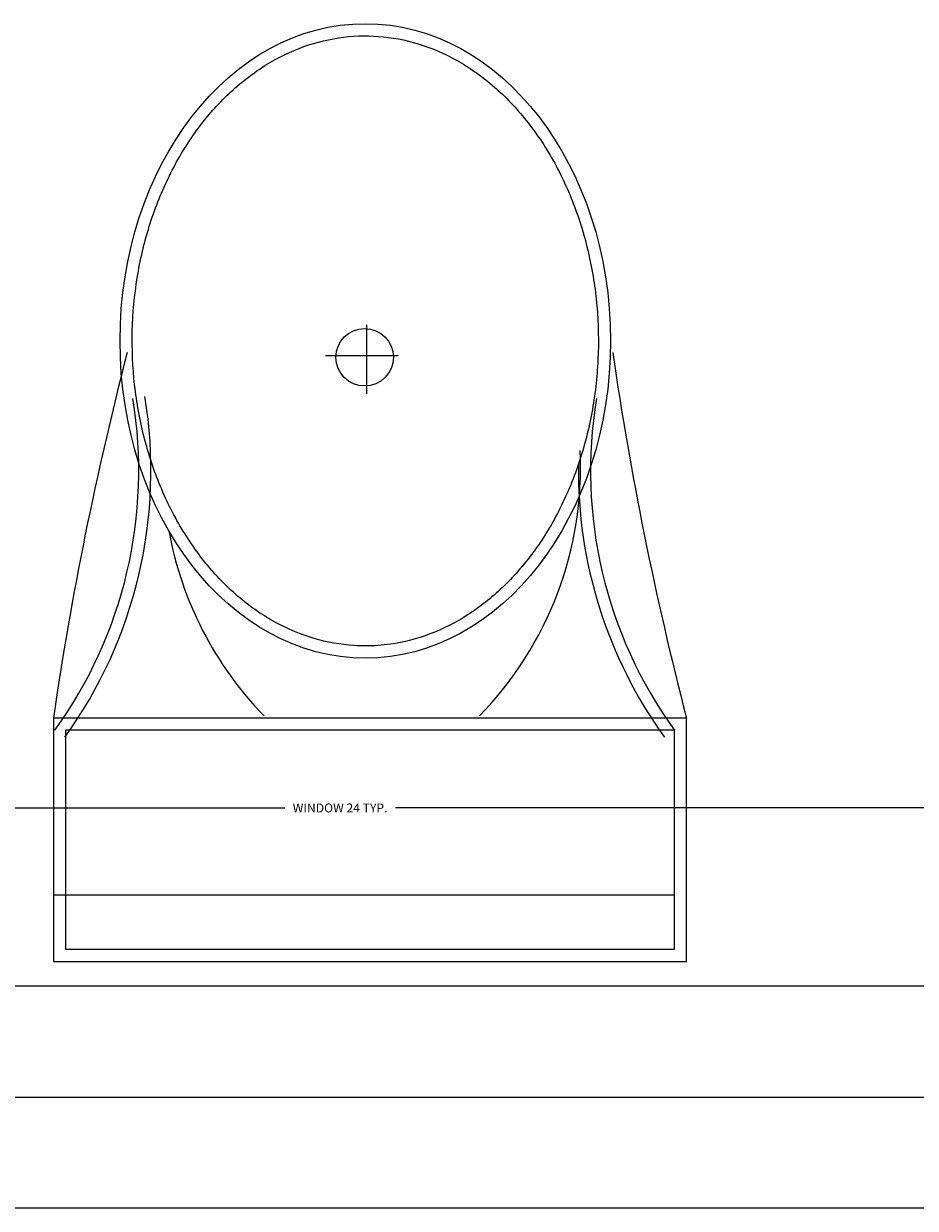
# Model space of a CAD drawing. Units: inches. Extents: x 1885 to 2748, y 783 to 2421.
# Tile 17 of 117: x 2125.82 to 2143.85, y 1087.51 to 1111.48. Entities that reach past the tile are written whole.
import ezdxf

# ---------------------------------------------------------------- set-up
doc = ezdxf.new("R2010")
doc.units = ezdxf.units.IN
for name, color, linetype, lineweight in [('A-ANNO-DIMS', 2, 'Continuous', 18), ('A-FLOR-FIXT', 8, 'Continuous', 18), ('A-GLAZ', 181, 'Continuous', 18)]:
    doc.layers.add(name, color=color, linetype=linetype, lineweight=lineweight)
doc.styles.get("Standard").update_dxf_attribs({"font": 'arial.ttf'})
doc.dimstyles.get("Standard").update_dxf_attribs({"dimtxt": 0.18, "dimasz": 0.18, "dimexe": 0.18, "dimexo": 0.0625, "dimgap": 0.09, "dimtad": 0, "dimtih": 1, "dimtoh": 1, "dimdec": 4, "dimzin": 0, "dimdsep": 46, "dimtxsty": 'Standard', "dimcen": 0.09, "dimadec": 0, "dimazin": 0, "dimtfac": 1, "dimtdec": 4, "dimtofl": 0, "dimtmove": 0, "dimatfit": 3, "dimfxl": 1, "dimtolj": 1, "dimtzin": 0, "dimarcsym": 0})

# ---------------------------------------------------------------- blocks, each defined once
blk = doc.blocks.new('A$C31115884')
for p, q in [((257.52, 466.4), (257.52, 523.22)), ((283.13, 497.65), (223.38, 497.65)), ((0, 200), (0, 0)), ((520, 200), (0, 200)), ((520, 0), (520, 200)), ((10, 190), (10, 10)), ((510, 190), (10, 190)), ((510, 10), (510, 190)), ((510, 54.46), (0, 54.46)), ((10, 10), (510, 10)), ((0, 0), (520, 0))]:
    blk.add_line(p, q)
blk.add_circle((255.63, 496.45), 23.6)
for centre, radius, start, end in [((2777.7, -204.57), 2807.01, 165.4549, 171.71327), ((3237.04, 904.96), 2807.01, 188.28673, 194.5451), ((-294.54, 403.26), 364.66, 324.20913, 9.34987), ((-294.54, 403.26), 374.66, 324.20913, 9.34987), ((805.79, 403.26), 364.66, 170.65013, 215.79087), ((139.48, 406.23), 293.48, 315.84364, 2.65635), ((805.79, 403.26), 374.66, 179.20365, 215.79087), ((383.57, 406.23), 293.48, 190.27735, 224.15636)]:
    blk.add_arc(centre, radius, start, end)
blk.add_ellipse((256.16, 509.9), major_axis=(0, -260.67), ratio=0.772727)
blk.add_open_spline([(256.16, 259.23), (263.08, 259.23), (269.99, 259.72), (287.81, 262.27), (298.65, 265.08), (319.86, 273.12), (330.22, 278.35), (350.15, 291.13), (359.72, 298.67), (377.75, 315.86), (386.21, 325.51), (401.75, 346.63), (408.82, 358.1), (421.35, 382.52), (426.79, 395.46), (435.87, 422.42), (439.5, 436.43), (444.83, 465.08), (446.52, 479.72), (447.92, 509.17), (447.62, 523.97), (445.03, 553.27), (442.74, 567.77), (436.26, 596.01), (432.07, 609.74), (421.91, 636.02), (415.95, 648.56), (402.47, 672.06), (394.95, 683.02), (378.6, 703.01), (369.78, 712.05), (351.11, 727.96), (341.27, 734.82), (320.89, 746.2), (310.35, 750.71), (288.88, 757.29), (277.96, 759.35), (256, 760.98), (244.98, 760.56), (223.13, 757.22), (212.3, 754.31), (191.14, 746.06), (180.8, 740.72), (160.94, 727.75), (151.41, 720.12), (133.48, 702.75), (125.07, 693.02), (109.65, 671.74), (102.63, 660.2), (90.25, 635.66), (84.88, 622.67), (75.95, 595.62), (72.4, 581.57), (67.24, 552.87), (65.63, 538.21), (64.4, 508.76), (64.79, 493.96), (67.54, 464.68), (69.91, 450.2), (76.56, 422.03), (80.83, 408.34), (91.13, 382.16), (97.16, 369.68), (110.77, 346.32), (118.35, 335.44), (134.81, 315.6), (143.69, 306.65), (162.44, 290.93), (172.32, 284.16), (192.75, 272.98), (203.31, 268.57), (224.81, 262.2), (235.75, 260.25), (249.87, 259.33), (253.02, 259.23), (256.16, 259.23)], degree=3, knots=[0, 0, 0, 0, 0.110105, 0.110105, 0.285049, 0.285049, 0.459994, 0.459994, 0.634938, 0.634938, 0.809882, 0.809882, 0.984827, 0.984827, 1.159771, 1.159771, 1.334715, 1.334715, 1.50966, 1.50966, 1.684604, 1.684604, 1.859549, 1.859549, 2.034493, 2.034493, 2.209437, 2.209437, 2.384382, 2.384382, 2.559326, 2.559326, 2.73427, 2.73427, 2.909215, 2.909215, 3.084159, 3.084159, 3.259103, 3.259103, 3.434048, 3.434048, 3.608992, 3.608992, 3.783936, 3.783936, 3.958881, 3.958881, 4.133825, 4.133825, 4.30877, 4.30877, 4.483714, 4.483714, 4.658658, 4.658658, 4.833603, 4.833603, 5.008547, 5.008547, 5.183491, 5.183491, 5.358436, 5.358436, 5.53338, 5.53338, 5.708324, 5.708324, 5.883269, 5.883269, 6.058213, 6.058213, 6.233158, 6.233158, 6.283185, 6.283185, 6.283185, 6.283185])
blk = doc.blocks.new('WIN-24')
for p, q in [((0.001, 4.496), (0.001, -0.004)), ((0.001, 4.496), (24.001, 4.496)), ((24.001, 2.246), (24.001, 4.496)), ((24.001, 4.496), (24.001, -0.004)), ((0.001, -0.004), (0.001, 2.246)), ((0.001, 2.246), (24.001, 2.246)), ((24.001, -0.004), (0.001, -0.004))]:
    blk.add_line(p, q)
blk = doc.blocks.new('*D23')
at = {"layer": 'A-ANNO-DIMS', "color": 0, "lineweight": -2, "transparency": 16777216}
for p, q in [((2120.221, 1092.068), (2120.221, 1095.786)), ((2144.221, 1092.068), (2144.221, 1095.786)), ((2120.401, 1095.606), (2131.102, 1095.606)), ((2144.041, 1095.606), (2133.339, 1095.606))]:
    blk.add_line(p, q, dxfattribs=at)
at = {"layer": 'A-ANNO-DIMS', "color": 0, "transparency": 16777216}
for points in [[(2120.401, 1095.636), (2120.401, 1095.576), (2120.221, 1095.606)], [(2144.041, 1095.636), (2144.041, 1095.576), (2144.221, 1095.606)]]:
    blk.add_solid(points, dxfattribs=at)
at = {"layer": 'Defpoints', "color": 0, "transparency": 16777216}
for p in [(2144.221, 1095.606), (2120.221, 1092.006), (2144.221, 1092.006)]:
    blk.add_point(p, dxfattribs=at)
at = {"layer": 'A-ANNO-DIMS', "color": 0, "transparency": 16777216, "insert": (2132.221, 1095.606), "char_height": 0.18, "attachment_point": 5}
blk.add_mtext('\\A1;WINDOW 24 TYP.', dxfattribs=at)

msp = doc.modelspace()

# ---------------------------------------------------------------- block references
at = {"layer": 'A-FLOR-FIXT', "xscale": 0.0246256636748975, "yscale": 0.0246256636748975, "zscale": 0.0246256636748975}
msp.add_blockref('A$C31115884', (2126.422, 1092.501), dxfattribs=at)
at = {"layer": 'A-GLAZ'}
msp.add_blockref('WIN-24', (2120.22, 1087.51), dxfattribs=at)

# ---------------------------------------------------------------- dimensions: what is measured, and where the dimension line sits
at = {"layer": 'A-ANNO-DIMS'}
dim = msp.add_linear_dim(base=(2144.221, 1095.606), p1=(2120.221, 1092.006), p2=(2144.221, 1092.006), text='WINDOW <> TYP.', dimstyle='Standard', override={"dimdec": 0, "dimlfac": 1, "dimrnd": 0, "dimzin": 0, "dimdsep": 46, "dimlunit": 2}, dxfattribs=at)
dim.commit()
dim.dimension.update_dxf_attribs({"geometry": '*D23', "text_midpoint": (2132.221, 1095.606)})

doc.saveas('drawing.dxf')
